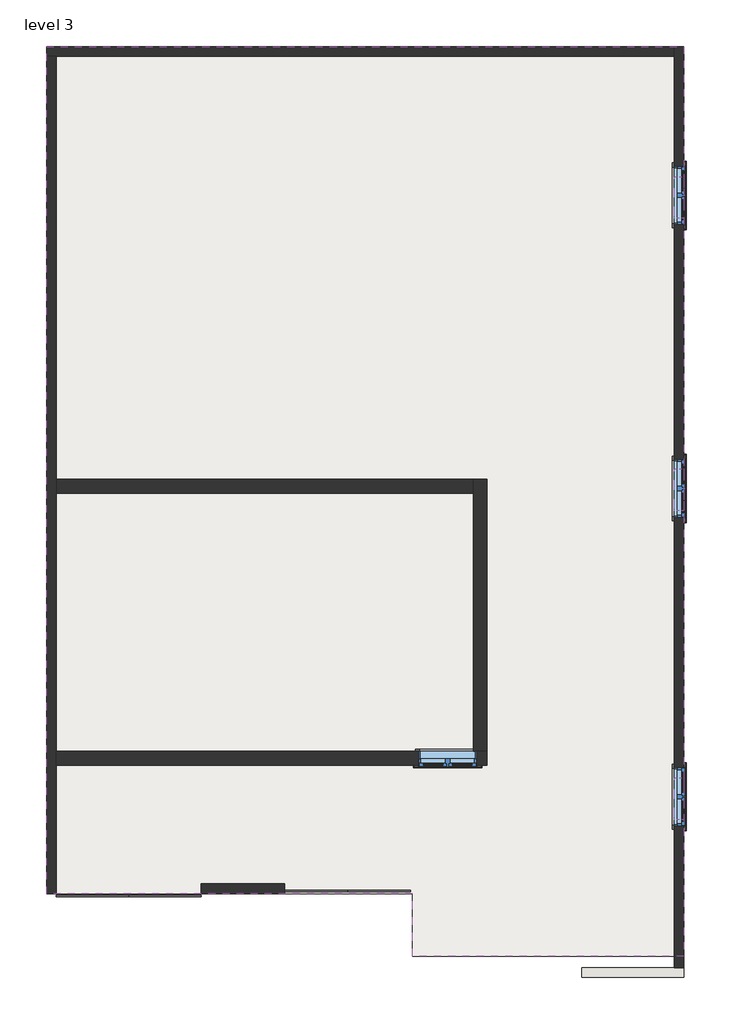
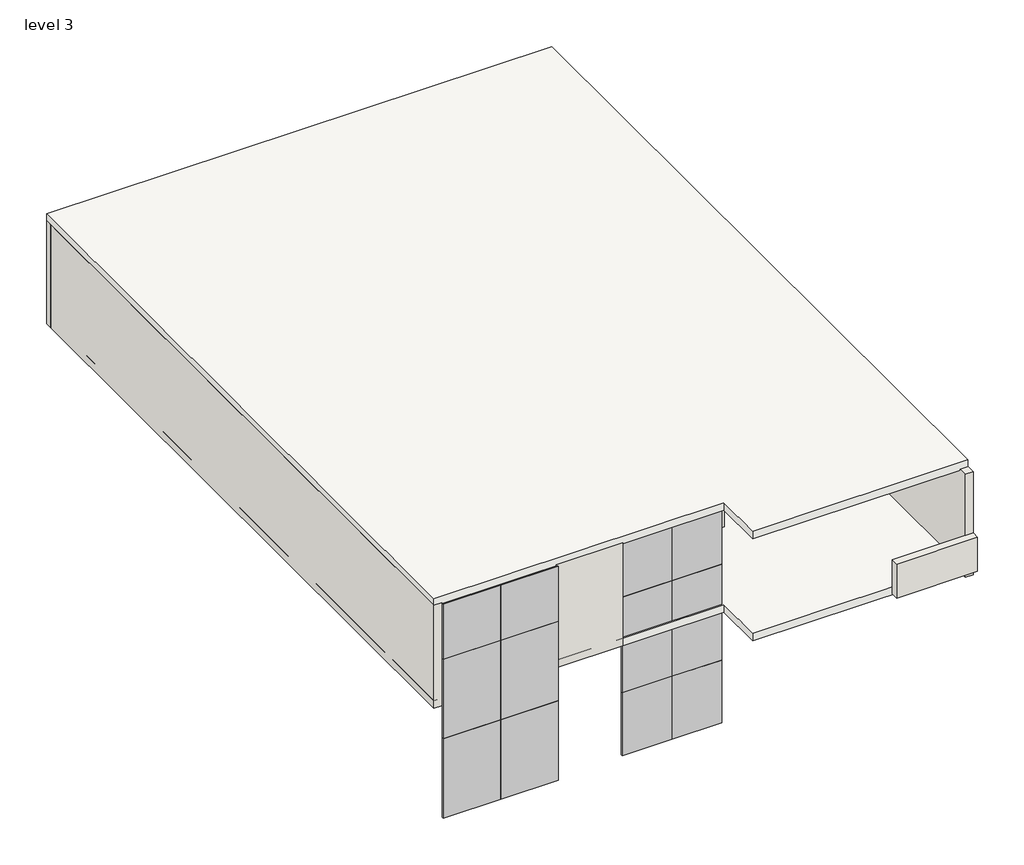
# One storey: 16 proxies, 12 plates, 8 walls, 7 windows, 2 slabs.
"""IFC4 building model written with IfcOpenShell, lengths in millimetres."""

from ifc_helpers import new_model, si_unit, frame, origin, place, context, project, spatial, polyline, outline, extrude, faceted_brep, transform, mapped, element, save
from components import m_muntin_pattern_2x2_m_muntin_pattern_2x2_62480ac4, m_muntin_pattern_2x2_m_muntin_pattern_2x2_4fd78f17, m_trim_window_exterior_flat_with_sill_90d3a428, m_trim_window_interior_flat_picture_frame_6ca9b1f8, system_panel_glazed_bea6ef26, system_panel_glazed_c442566e, system_panel_glazed_74a1dbaf, system_panel_glazed_90453812, system_panel_glazed_85540d86, m_fixed_0406_x_0610mm_8d3231a3, m_window_casement_double_850_x_900mm_0f766704, m_window_casement_double_850_x_900mm_77c4388a

model = new_model("IFC4")

# Units and contexts
model_context = context("Model", 3, world=origin())
ifc_project = project(units=[si_unit("LENGTHUNIT", "METRE", prefix="MILLI")], contexts=[model_context])

# Site, building, storey
site = spatial("IfcSite", under=ifc_project)
building = spatial("IfcBuilding", under=site)
storey = spatial("IfcBuildingStorey", under=building, Name="level 3", Elevation=7000.0)

# Proxies
placement = place(None, origin())
m_muntin_pattern_2x2_m_muntin_pattern_2x2_shape = m_muntin_pattern_2x2_m_muntin_pattern_2x2_62480ac4(model_context)
element("IfcBuildingElementProxy", 1, Name="M_Muntin Pattern_2x2 : M_Muntin Pattern_2x2", ObjectType="M_Muntin Pattern_2x2 : M_Muntin Pattern_2x2", at=placement, inside=storey, context=model_context, shape_type="MappedRepresentation", body=[
    mapped(m_muntin_pattern_2x2_m_muntin_pattern_2x2_shape, transform((-5582.3542042, -3112.6046146, 7671.0330914), x_axis=(-1.0, 0.0, 0.0), y_axis=(0.0, -1.0, 0.0), z_axis=(0.0, 0.0, 1.0))),
])
element("IfcBuildingElementProxy", 2, Name="M_Muntin Pattern_2x2 : M_Muntin Pattern_2x2", ObjectType="M_Muntin Pattern_2x2 : M_Muntin Pattern_2x2", at=placement, inside=storey, context=model_context, shape_type="MappedRepresentation", body=[
    mapped(m_muntin_pattern_2x2_m_muntin_pattern_2x2_shape, transform((-2362.9917042, -3370.6171146, 7623.9567455), x_axis=(0.0, -1.0, 0.0), y_axis=(1.0, 0.0, 0.0), z_axis=(0.0, 0.0, 1.0))),
])
element("IfcBuildingElementProxy", 3, Name="M_Muntin Pattern_2x2 : M_Muntin Pattern_2x2", ObjectType="M_Muntin Pattern_2x2 : M_Muntin Pattern_2x2", at=placement, inside=storey, context=model_context, shape_type="MappedRepresentation", body=[
    mapped(m_muntin_pattern_2x2_m_muntin_pattern_2x2_shape, transform((-2362.9917042, 1117.8578854, 7623.9567455), x_axis=(0.0, -1.0, 0.0), y_axis=(1.0, 0.0, 0.0), z_axis=(0.0, 0.0, 1.0))),
])
element("IfcBuildingElementProxy", 4, Name="M_Muntin Pattern_2x2 : M_Muntin Pattern_2x2", ObjectType="M_Muntin Pattern_2x2 : M_Muntin Pattern_2x2", at=placement, inside=storey, context=model_context, shape_type="MappedRepresentation", body=[
    mapped(m_muntin_pattern_2x2_m_muntin_pattern_2x2_shape, transform((-2362.9917042, 5385.0578854, 7623.9567455), x_axis=(0.0, -1.0, 0.0), y_axis=(1.0, 0.0, 0.0), z_axis=(0.0, 0.0, 1.0))),
])
m_muntin_pattern_2x2_m_muntin_pattern_2x2_2_shape = m_muntin_pattern_2x2_m_muntin_pattern_2x2_4fd78f17(model_context)
element("IfcBuildingElementProxy", 5, Name="M_Muntin Pattern_2x2 : M_Muntin Pattern_2x2", ObjectType="M_Muntin Pattern_2x2 : M_Muntin Pattern_2x2", at=placement, inside=storey, context=model_context, shape_type="MappedRepresentation", body=[
    mapped(m_muntin_pattern_2x2_m_muntin_pattern_2x2_2_shape, transform((-6004.1792042, -3112.6046146, 7671.0330914), x_axis=(1.0, 0.0, 0.0), y_axis=(0.0, 1.0, 0.0), z_axis=(0.0, 0.0, 1.0))),
])
element("IfcBuildingElementProxy", 6, Name="M_Muntin Pattern_2x2 : M_Muntin Pattern_2x2", ObjectType="M_Muntin Pattern_2x2 : M_Muntin Pattern_2x2", at=placement, inside=storey, context=model_context, shape_type="MappedRepresentation", body=[
    mapped(m_muntin_pattern_2x2_m_muntin_pattern_2x2_2_shape, transform((-2362.9917042, -3792.4421146, 7623.9567455), x_axis=(0.0, 1.0, 0.0), y_axis=(-1.0, 0.0, 0.0), z_axis=(0.0, 0.0, 1.0))),
])
element("IfcBuildingElementProxy", 7, Name="M_Muntin Pattern_2x2 : M_Muntin Pattern_2x2", ObjectType="M_Muntin Pattern_2x2 : M_Muntin Pattern_2x2", at=placement, inside=storey, context=model_context, shape_type="MappedRepresentation", body=[
    mapped(m_muntin_pattern_2x2_m_muntin_pattern_2x2_2_shape, transform((-2362.9917042, 696.0328854, 7623.9567455), x_axis=(0.0, 1.0, 0.0), y_axis=(-1.0, 0.0, 0.0), z_axis=(0.0, 0.0, 1.0))),
])
element("IfcBuildingElementProxy", 8, Name="M_Muntin Pattern_2x2 : M_Muntin Pattern_2x2", ObjectType="M_Muntin Pattern_2x2 : M_Muntin Pattern_2x2", at=placement, inside=storey, context=model_context, shape_type="MappedRepresentation", body=[
    mapped(m_muntin_pattern_2x2_m_muntin_pattern_2x2_2_shape, transform((-2362.9917042, 4963.2328854, 7623.9567455), x_axis=(0.0, 1.0, 0.0), y_axis=(-1.0, 0.0, 0.0), z_axis=(0.0, 0.0, 1.0))),
])
m_trim_window_exterior_flat_with_sill_shape = m_trim_window_exterior_flat_with_sill_90d3a428(model_context)
element("IfcBuildingElementProxy", 9, Name="M_Trim-Window-Exterior-Flat : with Sill", ObjectType="M_Trim-Window-Exterior-Flat : with Sill", at=placement, inside=storey, context=model_context, shape_type="MappedRepresentation", body=[
    mapped(m_trim_window_exterior_flat_with_sill_shape, transform((-5793.2667042, -3122.1296146, 8501.1830914), x_axis=(1.0, 0.0, 0.0), y_axis=(0.0, 0.0, 1.0), z_axis=(0.0, -1.0, 0.0))),
])
element("IfcBuildingElementProxy", 10, Name="M_Trim-Window-Exterior-Flat : with Sill", ObjectType="M_Trim-Window-Exterior-Flat : with Sill", at=placement, inside=storey, context=model_context, shape_type="MappedRepresentation", body=[
    mapped(m_trim_window_exterior_flat_with_sill_shape, transform((-2353.4667042, -3581.5296146, 8454.1067455), x_axis=(0.0, 1.0, 0.0), y_axis=(0.0, 0.0, 1.0), z_axis=(1.0, 0.0, 0.0))),
])
element("IfcBuildingElementProxy", 11, Name="M_Trim-Window-Exterior-Flat : with Sill", ObjectType="M_Trim-Window-Exterior-Flat : with Sill", at=placement, inside=storey, context=model_context, shape_type="MappedRepresentation", body=[
    mapped(m_trim_window_exterior_flat_with_sill_shape, transform((-2353.4667042, 906.9453854, 8454.1067455), x_axis=(0.0, 1.0, 0.0), y_axis=(0.0, 0.0, 1.0), z_axis=(1.0, 0.0, 0.0))),
])
element("IfcBuildingElementProxy", 12, Name="M_Trim-Window-Exterior-Flat : with Sill", ObjectType="M_Trim-Window-Exterior-Flat : with Sill", at=placement, inside=storey, context=model_context, shape_type="MappedRepresentation", body=[
    mapped(m_trim_window_exterior_flat_with_sill_shape, transform((-2353.4667042, 5174.1453854, 8454.1067455), x_axis=(0.0, 1.0, 0.0), y_axis=(0.0, 0.0, 1.0), z_axis=(1.0, 0.0, 0.0))),
])
m_trim_window_interior_flat_picture_frame_shape = m_trim_window_interior_flat_picture_frame_6ca9b1f8(model_context)
element("IfcBuildingElementProxy", 13, Name="M_Trim-Window-Interior-Flat : Picture Frame", ObjectType="M_Trim-Window-Interior-Flat : Picture Frame", at=placement, inside=storey, context=model_context, shape_type="MappedRepresentation", body=[
    mapped(m_trim_window_interior_flat_picture_frame_shape, transform((-5793.2667042, -2922.1296146, 8501.1830914), x_axis=(-1.0, 0.0, 0.0), y_axis=(0.0, 0.0, 1.0), z_axis=(0.0, 1.0, 0.0))),
])
element("IfcBuildingElementProxy", 14, Name="M_Trim-Window-Interior-Flat : Picture Frame", ObjectType="M_Trim-Window-Interior-Flat : Picture Frame", at=placement, inside=storey, context=model_context, shape_type="MappedRepresentation", body=[
    mapped(m_trim_window_interior_flat_picture_frame_shape, transform((-2493.4667042, -3581.5296146, 8454.1067455), x_axis=(0.0, -1.0, 0.0), y_axis=(0.0, 0.0, 1.0), z_axis=(-1.0, 0.0, 0.0))),
])
element("IfcBuildingElementProxy", 15, Name="M_Trim-Window-Interior-Flat : Picture Frame", ObjectType="M_Trim-Window-Interior-Flat : Picture Frame", at=placement, inside=storey, context=model_context, shape_type="MappedRepresentation", body=[
    mapped(m_trim_window_interior_flat_picture_frame_shape, transform((-2493.4667042, 906.9453854, 8454.1067455), x_axis=(0.0, -1.0, 0.0), y_axis=(0.0, 0.0, 1.0), z_axis=(-1.0, 0.0, 0.0))),
])
element("IfcBuildingElementProxy", 16, Name="M_Trim-Window-Interior-Flat : Picture Frame", ObjectType="M_Trim-Window-Interior-Flat : Picture Frame", at=placement, inside=storey, context=model_context, shape_type="MappedRepresentation", body=[
    mapped(m_trim_window_interior_flat_picture_frame_shape, transform((-2493.4667042, 5174.1453854, 8454.1067455), x_axis=(0.0, -1.0, 0.0), y_axis=(0.0, 0.0, 1.0), z_axis=(-1.0, 0.0, 0.0))),
])

# Plates
system_panel_glazed_shape = system_panel_glazed_bea6ef26(model_context)
element("IfcPlate", 17, ObjectType="System Panel : Glazed", at=placement, inside=storey, context=model_context, shape_type="MappedRepresentation", body=[
    mapped(system_panel_glazed_shape, transform((-9913.4667042, -4990.9296146, 7933.2), x_axis=(-1.0, 0.0, 0.0), y_axis=(0.0, -1.0, 0.0), z_axis=(0.0, 0.0, 1.0))),
])
element("IfcPlate", 18, ObjectType="System Panel : Glazed", at=placement, inside=storey, context=model_context, shape_type="MappedRepresentation", body=[
    mapped(system_panel_glazed_shape, transform((-10969.4667042, -4990.9296146, 7933.2), x_axis=(-1.0, 0.0, 0.0), y_axis=(0.0, -1.0, 0.0), z_axis=(0.0, 0.0, 1.0))),
])
system_panel_glazed_2_shape = system_panel_glazed_c442566e(model_context)
element("IfcPlate", 19, ObjectType="System Panel : Glazed", at=placement, inside=storey, context=model_context, shape_type="MappedRepresentation", body=[
    mapped(system_panel_glazed_2_shape, transform((-7709.0667042, -4990.9296146, 7933.2), x_axis=(1.0, 0.0, 0.0), y_axis=(0.0, 1.0, 0.0), z_axis=(0.0, 0.0, 1.0))),
])
element("IfcPlate", 20, ObjectType="System Panel : Glazed", at=placement, inside=storey, context=model_context, shape_type="MappedRepresentation", body=[
    mapped(system_panel_glazed_2_shape, transform((-6794.6667042, -4990.9296146, 7933.2), x_axis=(1.0, 0.0, 0.0), y_axis=(0.0, 1.0, 0.0), z_axis=(0.0, 0.0, 1.0))),
])
system_panel_glazed_3_shape = system_panel_glazed_74a1dbaf(model_context)
element("IfcPlate", 21, ObjectType="System Panel : Glazed", at=placement, inside=storey, context=model_context, shape_type="MappedRepresentation", body=[
    mapped(system_panel_glazed_3_shape, transform((-9913.4667042, -4990.9296146, 4850.0), x_axis=(-1.0, 0.0, 0.0), y_axis=(0.0, -1.0, 0.0), z_axis=(0.0, 0.0, 1.0))),
])
element("IfcPlate", 22, ObjectType="System Panel : Glazed", at=placement, inside=storey, context=model_context, shape_type="MappedRepresentation", body=[
    mapped(system_panel_glazed_3_shape, transform((-10969.4667042, -4990.9296146, 4850.0), x_axis=(-1.0, 0.0, 0.0), y_axis=(0.0, -1.0, 0.0), z_axis=(0.0, 0.0, 1.0))),
])
element("IfcPlate", 23, ObjectType="System Panel : Glazed", at=placement, inside=storey, context=model_context, shape_type="MappedRepresentation", body=[
    mapped(system_panel_glazed_3_shape, transform((-9913.4667042, -4990.9296146, 6391.6), x_axis=(-1.0, 0.0, 0.0), y_axis=(0.0, -1.0, 0.0), z_axis=(0.0, 0.0, 1.0))),
])
element("IfcPlate", 24, ObjectType="System Panel : Glazed", at=placement, inside=storey, context=model_context, shape_type="MappedRepresentation", body=[
    mapped(system_panel_glazed_3_shape, transform((-10969.4667042, -4990.9296146, 6391.6), x_axis=(-1.0, 0.0, 0.0), y_axis=(0.0, -1.0, 0.0), z_axis=(0.0, 0.0, 1.0))),
])
system_panel_glazed_4_shape = system_panel_glazed_90453812(model_context)
element("IfcPlate", 25, ObjectType="System Panel : Glazed", at=placement, inside=storey, context=model_context, shape_type="MappedRepresentation", body=[
    mapped(system_panel_glazed_4_shape, transform((-7709.0667042, -4990.9296146, 4850.0), x_axis=(1.0, 0.0, 0.0), y_axis=(0.0, 1.0, 0.0), z_axis=(0.0, 0.0, 1.0))),
])
element("IfcPlate", 26, ObjectType="System Panel : Glazed", at=placement, inside=storey, context=model_context, shape_type="MappedRepresentation", body=[
    mapped(system_panel_glazed_4_shape, transform((-6794.6667042, -4990.9296146, 4850.0), x_axis=(1.0, 0.0, 0.0), y_axis=(0.0, 1.0, 0.0), z_axis=(0.0, 0.0, 1.0))),
])
system_panel_glazed_5_shape = system_panel_glazed_85540d86(model_context)
element("IfcPlate", 27, ObjectType="System Panel : Glazed", at=placement, inside=storey, context=model_context, shape_type="MappedRepresentation", body=[
    mapped(system_panel_glazed_5_shape, transform((-7709.0667042, -4990.9296146, 6069.2), x_axis=(1.0, 0.0, 0.0), y_axis=(0.0, 1.0, 0.0), z_axis=(0.0, 0.0, 1.0))),
])
element("IfcPlate", 28, ObjectType="System Panel : Glazed", at=placement, inside=storey, context=model_context, shape_type="MappedRepresentation", body=[
    mapped(system_panel_glazed_5_shape, transform((-6794.6667042, -4990.9296146, 6069.2), x_axis=(1.0, 0.0, 0.0), y_axis=(0.0, 1.0, 0.0), z_axis=(0.0, 0.0, 1.0))),
])

# Slabs
element("IfcSlab", 29, ObjectType="Generic 150mm", at=placement, inside=storey, context=model_context, shape_type="SweptSolid", body=[
    extrude(outline(polyline([(-2353.4667042, 7341.0703854), (-2353.4667042, -5905.3296146), (-6306.9843842, -5905.3296146), (-6306.9843842, -4990.9296146), (-11637.4667042, -4990.9296146), (-11637.4667042, 7341.0703854), (-2353.4667042, 7341.0703854)])), frame((0.0, 0.0, 7000.0), z_axis=(0.0, 0.0, 1.0), x_axis=(1.0, 0.0, 0.0)), (0.0, 0.0, 1.0), 150.0),
])
element("IfcSlab", 30, ObjectType="Generic 150mm", at=placement, inside=storey, context=model_context, shape_type="SweptSolid", body=[
    extrude(outline(polyline([(-2353.4667042, 7341.0703854), (-2353.4667042, -5905.3296146), (-6306.9843842, -5905.3296146), (-6306.9843842, -4990.9296146), (-11637.4667042, -4990.9296146), (-11637.4667042, 7341.0703854), (-2353.4667042, 7341.0703854)])), frame((0.0, 0.0, 8981.2), z_axis=(0.0, 0.0, 1.0), x_axis=(1.0, 0.0, 0.0)), (0.0, 0.0, 1.0), 150.0),
])

# Walls
element("IfcWall", 31, ObjectType="Generic - 140mm Masonry", at=placement, inside=storey, context=model_context, shape_type="Brep", body=[
    faceted_brep([(-2353.4667042, -6071.9259117, 7000.0), (-2353.4667042, 7341.0703854, 7000.0), (-2353.4667042, 7341.0703854, 9000.0), (-2353.4667042, -6071.9259117, 9000.0), (-2353.4667042, -6071.9259117, 7813.3686956), (-2353.4667042, -6071.9259117, 7150.0), (-2353.4667042, -4006.5296146, 8454.1067455), (-2353.4667042, -3156.5296146, 8454.1067455), (-2353.4667042, -3156.5296146, 7554.1067455), (-2353.4667042, -4006.5296146, 7554.1067455), (-2353.4667042, 481.9453854, 8454.1067455), (-2353.4667042, 1331.9453854, 8454.1067455), (-2353.4667042, 1331.9453854, 7554.1067455), (-2353.4667042, 481.9453854, 7554.1067455), (-2353.4667042, 4749.1453854, 8454.1067455), (-2353.4667042, 5599.1453854, 8454.1067455), (-2353.4667042, 5599.1453854, 7554.1067455), (-2353.4667042, 4749.1453854, 7554.1067455), (-2353.4667042, -3303.3259117, 8648.8718004), (-2353.4667042, -3912.9259117, 8648.8718004), (-2353.4667042, -3912.9259117, 8953.6718004), (-2353.4667042, -3303.3259117, 8953.6718004), (-2353.4667042, 1192.4740883, 8648.6603549), (-2353.4667042, 582.8740883, 8648.6603549), (-2353.4667042, 582.8740883, 8953.4603549), (-2353.4667042, 1192.4740883, 8953.4603549), (-2353.4667042, 5448.4703854, 8649.9699652), (-2353.4667042, 4838.8703854, 8649.9699652), (-2353.4667042, 4838.8703854, 8954.7699652), (-2353.4667042, 5448.4703854, 8954.7699652), (-2493.4667042, -6071.9259117, 7000.0), (-2493.4667042, -6071.9259117, 9000.0), (-2493.4667042, 7201.0703854, 9000.0), (-2493.4667042, 7341.0703854, 9000.0), (-2493.4667042, 7341.0703854, 7000.0), (-2493.4667042, 7201.0703854, 7000.0), (-2493.4667042, -4006.5296146, 8454.1067455), (-2493.4667042, -4006.5296146, 7554.1067455), (-2493.4667042, -3156.5296146, 7554.1067455), (-2493.4667042, -3156.5296146, 8454.1067455), (-2493.4667042, 481.9453854, 8454.1067455), (-2493.4667042, 481.9453854, 7554.1067455), (-2493.4667042, 1331.9453854, 7554.1067455), (-2493.4667042, 1331.9453854, 8454.1067455), (-2493.4667042, 4749.1453854, 8454.1067455), (-2493.4667042, 4749.1453854, 7554.1067455), (-2493.4667042, 5599.1453854, 7554.1067455), (-2493.4667042, 5599.1453854, 8454.1067455), (-2493.4667042, -3303.3259117, 8648.8718004), (-2493.4667042, -3303.3259117, 8953.6718004), (-2493.4667042, -3912.9259117, 8953.6718004), (-2493.4667042, -3912.9259117, 8648.8718004), (-2493.4667042, 1192.4740883, 8648.6603549), (-2493.4667042, 1192.4740883, 8953.4603549), (-2493.4667042, 582.8740883, 8953.4603549), (-2493.4667042, 582.8740883, 8648.6603549), (-2493.4667042, 5448.4703854, 8649.9699652), (-2493.4667042, 5448.4703854, 8954.7699652), (-2493.4667042, 4838.8703854, 8954.7699652), (-2493.4667042, 4838.8703854, 8649.9699652)], [[[0, 1, 2, 3, 4, 5], [6, 7, 8, 9], [10, 11, 12, 13], [14, 15, 16, 17], [18, 19, 20, 21], [22, 23, 24, 25], [26, 27, 28, 29]], [[30, 31, 32, 33, 34, 35], [36, 37, 38, 39], [40, 41, 42, 43], [44, 45, 46, 47], [48, 49, 50, 51], [52, 53, 54, 55], [56, 57, 58, 59]], [[1, 0, 30, 35, 34]], [[3, 2, 33, 32, 31]], [[2, 1, 34, 33]], [[0, 5, 4, 3, 31, 30]], [[37, 36, 6, 9]], [[38, 37, 9, 8]], [[39, 38, 8, 7]], [[36, 39, 7, 6]], [[41, 40, 10, 13]], [[42, 41, 13, 12]], [[43, 42, 12, 11]], [[40, 43, 11, 10]], [[45, 44, 14, 17]], [[46, 45, 17, 16]], [[47, 46, 16, 15]], [[44, 47, 15, 14]], [[49, 48, 18, 21]], [[50, 49, 21, 20]], [[51, 50, 20, 19]], [[48, 51, 19, 18]], [[53, 52, 22, 25]], [[54, 53, 25, 24]], [[55, 54, 24, 23]], [[52, 55, 23, 22]], [[57, 56, 26, 29]], [[58, 57, 29, 28]], [[59, 58, 28, 27]], [[56, 59, 27, 26]]]),
])
element("IfcWall", 32, ObjectType="Generic - 140mm Masonry", at=placement, inside=storey, context=model_context, shape_type="Brep", body=[
    faceted_brep([(-2493.4667042, 7341.0703854, 7000.0), (-11637.4667042, 7341.0703854, 7000.0), (-11637.4667042, 7341.0703854, 9000.0), (-2493.4667042, 7341.0703854, 9000.0), (-2493.4667042, 7201.0703854, 7000.0), (-2493.4667042, 7201.0703854, 9000.0), (-11497.4667042, 7201.0703854, 9000.0), (-11637.4667042, 7201.0703854, 9000.0), (-11637.4667042, 7201.0703854, 7000.0), (-11497.4667042, 7201.0703854, 7000.0)], [[[0, 1, 2, 3]], [[4, 5, 6, 7, 8, 9]], [[1, 0, 4, 9, 8]], [[3, 2, 7, 6, 5]], [[0, 3, 5, 4]], [[2, 1, 8, 7]]]),
])
element("IfcWall", 33, ObjectType="Generic - 140mm Masonry", at=placement, inside=storey, context=model_context, shape_type="Brep", body=[
    faceted_brep([(-11637.4667042, 7201.0703854, 7000.0), (-11637.4667042, -4990.9296146, 7000.0), (-11637.4667042, -4990.9296146, 9000.0), (-11637.4667042, 7201.0703854, 9000.0), (-11497.4667042, 7201.0703854, 7000.0), (-11497.4667042, 7201.0703854, 9000.0), (-11497.4667042, 1040.2703854, 9000.0), (-11497.4667042, 840.2703854, 9000.0), (-11497.4667042, -2922.1296146, 9000.0), (-11497.4667042, -3122.1296146, 9000.0), (-11497.4667042, -4990.9296146, 9000.0), (-11497.4667042, -4990.9296146, 7000.0), (-11497.4667042, -3122.1296146, 7000.0), (-11497.4667042, -2922.1296146, 7000.0), (-11497.4667042, 840.2703854, 7000.0), (-11497.4667042, 1040.2703854, 7000.0)], [[[0, 1, 2, 3]], [[4, 5, 6, 7, 8, 9, 10, 11, 12, 13, 14, 15]], [[1, 0, 4, 15, 14, 13, 12, 11]], [[2, 1, 11, 10]], [[3, 2, 10, 9, 8, 7, 6, 5]], [[0, 3, 5, 4]]]),
])
element("IfcWall", 34, ObjectType="Generic - 140mm Masonry", at=placement, inside=storey, context=model_context, shape_type="SweptSolid", body=[
    extrude(outline(polyline([(-2353.4667042, -6211.9259117), (-3838.1043842, -6211.9259117), (-3838.1043842, -6071.9259117), (-2353.4667042, -6071.9259117), (-2353.4667042, -6211.9259117)])), frame((0.0, 0.0, 7150.0), z_axis=(0.0, 0.0, 1.0), x_axis=(1.0, 0.0, 0.0)), (0.0, 0.0, 1.0), 663.3686956),
])
element("IfcWall", 35, ObjectType="Generic - 140mm Masonry", at=placement, inside=storey, context=model_context, shape_type="SweptSolid", body=[
    extrude(outline(polyline([(-8166.2667042, -4990.9296146), (-9385.4667042, -4990.9296146), (-9385.4667042, -4850.9296146), (-8166.2667042, -4850.9296146), (-8166.2667042, -4990.9296146)])), frame((0.0, 0.0, 7000.0), z_axis=(0.0, 0.0, 1.0), x_axis=(1.0, 0.0, 0.0)), (0.0, 0.0, 1.0), 2000.0),
])
element("IfcWall", 36, ObjectType="Generic - 200mm", at=placement, inside=storey, context=model_context, shape_type="Brep", body=[
    faceted_brep([(-11497.4667042, -3122.1296146, 7000.0), (-5219.0667042, -3122.1296146, 7000.0), (-5219.0667042, -3122.1296146, 9000.0), (-11497.4667042, -3122.1296146, 9000.0), (-6218.2667042, -3122.1296146, 8501.1830914), (-5368.2667042, -3122.1296146, 8501.1830914), (-5368.2667042, -3122.1296146, 7601.1830914), (-6218.2667042, -3122.1296146, 7601.1830914), (-11497.4667042, -2922.1296146, 7000.0), (-11497.4667042, -2922.1296146, 9000.0), (-5419.0667042, -2922.1296146, 9000.0), (-5219.0667042, -2922.1296146, 9000.0), (-5219.0667042, -2922.1296146, 7000.0), (-5419.0667042, -2922.1296146, 7000.0), (-6218.2667042, -2922.1296146, 8501.1830914), (-6218.2667042, -2922.1296146, 7601.1830914), (-5368.2667042, -2922.1296146, 7601.1830914), (-5368.2667042, -2922.1296146, 8501.1830914)], [[[0, 1, 2, 3], [4, 5, 6, 7]], [[8, 9, 10, 11, 12, 13], [14, 15, 16, 17]], [[1, 0, 8, 13, 12]], [[3, 2, 11, 10, 9]], [[0, 3, 9, 8]], [[2, 1, 12, 11]], [[15, 14, 4, 7]], [[16, 15, 7, 6]], [[17, 16, 6, 5]], [[14, 17, 5, 4]]]),
])
element("IfcWall", 37, ObjectType="Generic - 200mm", at=placement, inside=storey, context=model_context, shape_type="Brep", body=[
    faceted_brep([(-5219.0667042, -2922.1296146, 7000.0), (-5219.0667042, 1040.2703854, 7000.0), (-5219.0667042, 1040.2703854, 9000.0), (-5219.0667042, -2922.1296146, 9000.0), (-5419.0667042, -2922.1296146, 7000.0), (-5419.0667042, -2922.1296146, 9000.0), (-5419.0667042, 840.2703854, 9000.0), (-5419.0667042, 1040.2703854, 9000.0), (-5419.0667042, 1040.2703854, 7000.0), (-5419.0667042, 840.2703854, 7000.0)], [[[0, 1, 2, 3]], [[4, 5, 6, 7, 8, 9]], [[1, 0, 4, 9, 8]], [[3, 2, 7, 6, 5]], [[0, 3, 5, 4]], [[2, 1, 8, 7]]]),
])
element("IfcWall", 38, ObjectType="Generic - 200mm", at=placement, inside=storey, context=model_context, shape_type="SweptSolid", body=[
    extrude(outline(polyline([(-11497.4667042, 1040.2703854), (-5419.0667042, 1040.2703854), (-5419.0667042, 840.2703854), (-11497.4667042, 840.2703854), (-11497.4667042, 1040.2703854)])), frame((0.0, 0.0, 7000.0), z_axis=(0.0, 0.0, 1.0), x_axis=(1.0, 0.0, 0.0)), (0.0, 0.0, 1.0), 2000.0),
])

# Windows
m_fixed_0406_x_0610mm_shape = m_fixed_0406_x_0610mm_8d3231a3(model_context)
element("IfcWindow", 39, ObjectType="M_Fixed : 0406 x 0610mm", at=placement, inside=storey, context=model_context, shape_type="MappedRepresentation", body=[
    mapped(m_fixed_0406_x_0610mm_shape, transform((-2436.4667042, -3608.1259117, 7733.8718004), x_axis=(0.0, -1.0, 0.0), y_axis=(1.0, 0.0, 0.0), z_axis=(0.0, 0.0, 1.0))),
])
element("IfcWindow", 40, ObjectType="M_Fixed : 0406 x 0610mm", at=placement, inside=storey, context=model_context, shape_type="MappedRepresentation", body=[
    mapped(m_fixed_0406_x_0610mm_shape, transform((-2436.4667042, 887.6740883, 7733.6603549), x_axis=(0.0, -1.0, 0.0), y_axis=(1.0, 0.0, 0.0), z_axis=(0.0, 0.0, 1.0))),
])
element("IfcWindow", 41, ObjectType="M_Fixed : 0406 x 0610mm", at=placement, inside=storey, context=model_context, shape_type="MappedRepresentation", body=[
    mapped(m_fixed_0406_x_0610mm_shape, transform((-2436.4667042, 5143.6703854, 7734.9699652), x_axis=(0.0, -1.0, 0.0), y_axis=(1.0, 0.0, 0.0), z_axis=(0.0, 0.0, 1.0))),
])
m_window_casement_double_850_x_900mm_shape = m_window_casement_double_850_x_900mm_0f766704(model_context)
element("IfcWindow", 42, ObjectType="M_Window-Casement-Double : 850 x 900mm", at=placement, inside=storey, context=model_context, shape_type="MappedRepresentation", body=[
    mapped(m_window_casement_double_850_x_900mm_shape, transform((-5793.2667042, -3022.1296146, 6701.1830914), x_axis=(-1.0, 0.0, 0.0), y_axis=(0.0, -1.0, 0.0), z_axis=(0.0, 0.0, 1.0))),
])
m_window_casement_double_850_x_900mm_2_shape = m_window_casement_double_850_x_900mm_77c4388a(model_context)
element("IfcWindow", 43, ObjectType="M_Window-Casement-Double : 850 x 900mm", at=placement, inside=storey, context=model_context, shape_type="MappedRepresentation", body=[
    mapped(m_window_casement_double_850_x_900mm_2_shape, transform((-2423.4667042, -3581.5296146, 6654.1067455), x_axis=(0.0, -1.0, 0.0), y_axis=(1.0, 0.0, 0.0), z_axis=(0.0, 0.0, 1.0))),
])
element("IfcWindow", 44, ObjectType="M_Window-Casement-Double : 850 x 900mm", at=placement, inside=storey, context=model_context, shape_type="MappedRepresentation", body=[
    mapped(m_window_casement_double_850_x_900mm_2_shape, transform((-2423.4667042, 906.9453854, 6654.1067455), x_axis=(0.0, -1.0, 0.0), y_axis=(1.0, 0.0, 0.0), z_axis=(0.0, 0.0, 1.0))),
])
element("IfcWindow", 45, ObjectType="M_Window-Casement-Double : 850 x 900mm", at=placement, inside=storey, context=model_context, shape_type="MappedRepresentation", body=[
    mapped(m_window_casement_double_850_x_900mm_2_shape, transform((-2423.4667042, 5174.1453854, 6654.1067455), x_axis=(0.0, -1.0, 0.0), y_axis=(1.0, 0.0, 0.0), z_axis=(0.0, 0.0, 1.0))),
])

save(model, "model.ifc")

# Revit data of these elements
# Type "M_Muntin Pattern_2x2 : M_Muntin Pattern_2x2"
#   Width [instance default] = 3.937008 ft
#   Thickness = 0.041667 ft
#   Height [instance default] = 3.937008 ft
#   Distance = 0.0625 ft
#   Interior Material [instance default] = none
#   Exterior Material [instance default] = none
#   Default Elevation = 0
# Type "M_Trim-Window-Exterior-Flat : with Sill"
#   Trim Width = 0.19685 ft
#   Trim Thickness_Picture Frame = 0.098425 ft
#   Trim Thickness_with Sill = 0.0625 ft
#   Sill Thickness = 0.098425 ft
#   Opening Width [instance default] = 1.968504 ft
#   Opening Height [instance default] = 2.952756 ft
#   Default Elevation = 3.937008 ft
#   Sill = yes
#   Picture Frame = no
#   Trim Material [instance default] = none
# Type "M_Trim-Window-Interior-Flat : Picture Frame"
#   Trim Thickness_Picture Frame = 0.098425 ft
#   Trim Width = 0.19685 ft
#   Trim Thickness_with Sill = 0.065617 ft
#   Sill Thickness = 0.098425 ft
#   Opening Width [instance default] = 1.968504 ft
#   Opening Height [instance default] = 2.952756 ft
#   Default Elevation = 3.937008 ft
#   Sill = no
#   Picture Frame = yes
#   Trim Material [instance default] = none
# Type "System Panel : Glazed"
#   Construction Type Id = "GSP4R"
#   Analytic Construction = "1/8 in Pilkington single glazing"
#   Visual Light Transmittance = 0.9
#   Solar Heat Gain Coefficient = 0.86
#   Heat Transfer Coefficient (U) = 6.7069 W/(m²·K)
#   Define Thermal Properties by = 1
# Type "Generic 150mm"
#   Function = 0
#   Layers, outside or top first: 0.492126 ft no material (function 1)
# Type "Generic - 140mm Masonry"
#   Layers, outside or top first: 0.459318 ft "Concrete Masonry Units" (function 1)
# Type "Generic - 200mm"
#   Layers, outside or top first: 0.656168 ft no material (function 1)
# Type "M_Fixed : 0406 x 0610mm"
#   Type Mark = "10"
#   Construction Type Id = "GSP4R"
#   Analytic Construction = "1/8 in Pilkington single glazing"
#   Visual Light Transmittance = 0.9
#   Thermal Resistance (R) = 0.271106 (m²·K)/W
#   Solar Heat Gain Coefficient = 0.78
#   Heat Transfer Coefficient (U) = 3.6886 W/(m²·K)
#   Height = 1 ft
#   Default Sill Height = 3.001969 ft
#   Width = 2 ft
#   Window Inset = 0.062336 ft
#   Define Thermal Properties by = 1
#   Define Thermal Properties by = 1
#   Frame Exterior Material = Sash
#   Frame Interior Material = Sash
#   Glass Pane Material = Glass
#   Sash = Sash
#   Wall Closure = (empty or 0)
# Type "M_Window-Casement-Double : 850 x 900mm"
#   Type Mark = "23"
#   Fire Rating = "0.5h"
#   Assembly Code = "B2020100"
#   Analytic Construction = "Double glazing - domestic"
#   Frame Extension [instance default] = 0.020833 ft
#   Window Inset [instance default] = 0 ft
#   Wall Thickness [instance default] = 0.492126 ft
#   Interior Wall Closure [instance default] = 0.179626 ft
#   Half Width = 1.394357 ft
#   Visual Light Transmittance = 0.81
#   Thermal Resistance (R) = 0.319569 (m²·K)/W
#   Solar Heat Gain Coefficient = 0.76
#   Rough Width = 2.837927 ft
#   Rough Height = 3.001969 ft
#   Height = 2.952756 ft
#   Heat Transfer Coefficient (U) = 3.12929 W/(m²·K)
#   Exterior Wall Closure [instance default] = 0.104331 ft
#   Extension Jamb [instance default] = 0.179626 ft
#   Default Sill Height = 2.952756 ft
#   Width = 2.788714 ft
#   Define Thermal Properties by = 0
#   Muntin Visibility = yes
#   Interior Trim Visibility [instance default] = yes
#   Exterior Trim Visibility [instance default] = yes
#   Extension Jamb Visibility [instance default] = yes
#   Interior Trim Material = Wood - Stained
#   Muntin Pattern = M_Muntin Pattern_2x2 : M_Muntin Pattern_2x2
#   Interior Trim = M_Trim-Window-Interior-Flat : Picture Frame
#   Interior Frame Material = Wood - Stained
#   Glass Panel Material = Glass
#   Exterior Trim Material = Clad - White
#   Exterior Trim = M_Trim-Window-Exterior-Flat : with Sill
#   Exterior Frame Material = Clad - White
#   Wall Closure = (empty or 0)
# Elements 1, 2, 3, 4, 5, 6, 7, 8 (IfcBuildingElementProxy, "M_Muntin Pattern_2x2 : M_Muntin Pattern_2x2")
#   Width = 0.94644 ft
#   Height = 2.494423 ft
#   Interior Material = Wood - Stained
#   Exterior Material = Clad - White
#   Phase Created = New Construction
#   Materials on its faces: "Clad - White", "Wood - Stained"
# Elements 9, 10, 11, 12 (IfcBuildingElementProxy, "M_Trim-Window-Exterior-Flat : with Sill")
#   Opening Width = 2.788714 ft
#   Opening Height = 2.952756 ft
#   Trim Material = Clad - White
#   Phase Created = New Construction
#   Materials on its faces: "Clad - White"
# Elements 13, 14, 15, 16 (IfcBuildingElementProxy, "M_Trim-Window-Interior-Flat : Picture Frame")
#   Opening Width = 2.788714 ft
#   Opening Height = 2.952756 ft
#   Trim Material = Wood - Stained
#   Phase Created = New Construction
#   Materials on its faces: "Wood - Stained"
# Elements 17, 18, 19, 20, 21, 22, 23, 24, 25, 26, 27, 28 (IfcPlate, "System Panel : Glazed")
#   Phase Created = New Construction
#   Materials on its faces: "Glass"
# Element 29 (IfcSlab, "Generic 150mm")
#   Height Offset From Level = 0.492126 ft
#   Phase Created = New Construction
#   Materials on its faces: "Default Floor"
# Element 30 (IfcSlab, "Generic 150mm")
#   Height Offset From Level = 6.992126 ft
#   Phase Created = New Construction
#   Materials on its faces: "Default Floor"
# Element 31 (IfcWall, "Generic - 140mm Masonry")
#   Top Offset = 6.56168 ft
#   Base Offset = 0 ft
#   wall height = 6.56168 ft
#   Phase Created = New Construction
#   Base Constraint = level 3
#   Top Constraint = level 3
#   Materials on its faces: "Concrete Masonry Units", "Cherry", "YELLOW"
# Element 32 (IfcWall, "Generic - 140mm Masonry")
#   Top Offset = 6.56168 ft
#   Base Offset = 0 ft
#   wall height = 6.56168 ft
#   Phase Created = New Construction
#   Base Constraint = level 3
#   Top Constraint = level 3
#   Materials on its faces: "Concrete Masonry Units", "PAINT", "Cherry"
# Element 33 (IfcWall, "Generic - 140mm Masonry")
#   Top Offset = 6.56168 ft
#   Base Offset = 0 ft
#   wall height = 6.56168 ft
#   Phase Created = New Construction
#   Base Constraint = level 3
#   Top Constraint = level 3
#   Materials on its faces: "Concrete Masonry Units", "Cherry", "PAINT"
# Element 34 (IfcWall, "Generic - 140mm Masonry")
#   built-in parameter 1001111 = 0.492126 ft
#   Top Offset = 0 ft
#   Base Offset = 0.492126 ft
#   Unconnected Height = 2.176406 ft
#   wall height = 2.176406 ft
#   Phase Created = New Construction
#   Base Constraint = level 3
#   Materials on its faces: "Concrete Masonry Units", "Glass", "Cherry"
# Element 35 (IfcWall, "Generic - 140mm Masonry")
#   Top Offset = 6.56168 ft
#   Base Offset = 0 ft
#   wall height = 6.56168 ft
#   Phase Created = New Construction
#   Base Constraint = level 3
#   Top Constraint = level 3
#   Materials on its faces: "Concrete Masonry Units", "Clad - White"
# Element 36 (IfcWall, "Generic - 200mm")
#   Top Offset = 0 ft
#   Base Offset = 0 ft
#   Unconnected Height = 6.56168 ft
#   wall height = 6.56168 ft
#   Phase Created = New Construction
#   Base Constraint = level 3
#   Materials on its faces: "Default Wall", "PAINT"
# Elements 37, 38 (IfcWall, "Generic - 200mm")
#   Top Offset = 0 ft
#   Base Offset = 0 ft
#   Unconnected Height = 6.56168 ft
#   wall height = 6.56168 ft
#   Phase Created = New Construction
#   Base Constraint = level 3
#   Materials on its faces: "Default Wall"
# Element 39 (IfcWindow, "M_Fixed : 0406 x 0610mm")
#   Mark = "23"
#   Phase Created = New Construction
#   Materials on its faces: "Sash", "Glass"
# Element 40 (IfcWindow, "M_Fixed : 0406 x 0610mm")
#   Mark = "24"
#   Phase Created = New Construction
#   Materials on its faces: "Sash", "Glass"
# Element 41 (IfcWindow, "M_Fixed : 0406 x 0610mm")
#   Mark = "27"
#   Phase Created = New Construction
#   Materials on its faces: "Sash", "Glass"
# Element 42 (IfcWindow, "M_Window-Casement-Double : 850 x 900mm")
#   Mark = "15"
#   Window Inset = 0 ft
#   Interior Wall Closure = 0.179626 ft
#   Frame Extension = 0.020833 ft
#   Exterior Wall Closure = 0.104331 ft
#   Interior Trim Visibility = yes
#   Exterior Trim Visibility = yes
#   Phase Created = New Construction
#   Materials on its faces: "Wood - Stained", "Glass", "Clad - White"
# Element 43 (IfcWindow, "M_Window-Casement-Double : 850 x 900mm")
#   Mark = "19"
#   Window Inset = 0 ft
#   Interior Wall Closure = 0.179626 ft
#   Frame Extension = 0.020833 ft
#   Exterior Wall Closure = 0.104331 ft
#   Interior Trim Visibility = yes
#   Exterior Trim Visibility = yes
#   Phase Created = New Construction
#   Materials on its faces: "Wood - Stained", "Glass", "Clad - White"
# Element 44 (IfcWindow, "M_Window-Casement-Double : 850 x 900mm")
#   Mark = "20"
#   Window Inset = 0 ft
#   Interior Wall Closure = 0.179626 ft
#   Frame Extension = 0.020833 ft
#   Exterior Wall Closure = 0.104331 ft
#   Interior Trim Visibility = yes
#   Exterior Trim Visibility = yes
#   Phase Created = New Construction
#   Materials on its faces: "Wood - Stained", "Glass", "Clad - White"
# Element 45 (IfcWindow, "M_Window-Casement-Double : 850 x 900mm")
#   Mark = "21"
#   Window Inset = 0 ft
#   Interior Wall Closure = 0.179626 ft
#   Frame Extension = 0.020833 ft
#   Exterior Wall Closure = 0.104331 ft
#   Interior Trim Visibility = yes
#   Exterior Trim Visibility = yes
#   Phase Created = New Construction
#   Materials on its faces: "Wood - Stained", "Glass", "Clad - White"
# Materials
#   "Concrete Masonry Units": class "Masonry", colour RGB 181 181 181, transparency 0, Description = "Concrete masonry units", Cost = 0
#   "Sash": class "Wood", colour RGB 224 178 126, transparency 0, Cost = 0
#   "Glass": class "Glass", colour RGB 0 128 192, transparency 0.9, Description = "Soda Lime Glass", Cost = 0
#   "Wood - Stained": class "Wood", colour RGB 224 178 126, transparency 0, Cost = 0
#   "Clad - White": class "Wood", colour RGB 242 242 238, transparency 0, Cost = 0
#   "Default Floor": colour RGB 127 127 127, transparency 0, Cost = 0
#   "Cherry": class "Wood", colour RGB 226 177 128, transparency 0, Description = "Prunus Serotina", Cost = 0
#   "YELLOW": class "Generic", colour RGB 255 255 0, transparency 0, Cost = 0
#   "PAINT": class "Generic", colour RGB 105 77 58, transparency 0, Cost = 0
#   "Default Wall": colour RGB 128 128 128, transparency 0, Cost = 0
